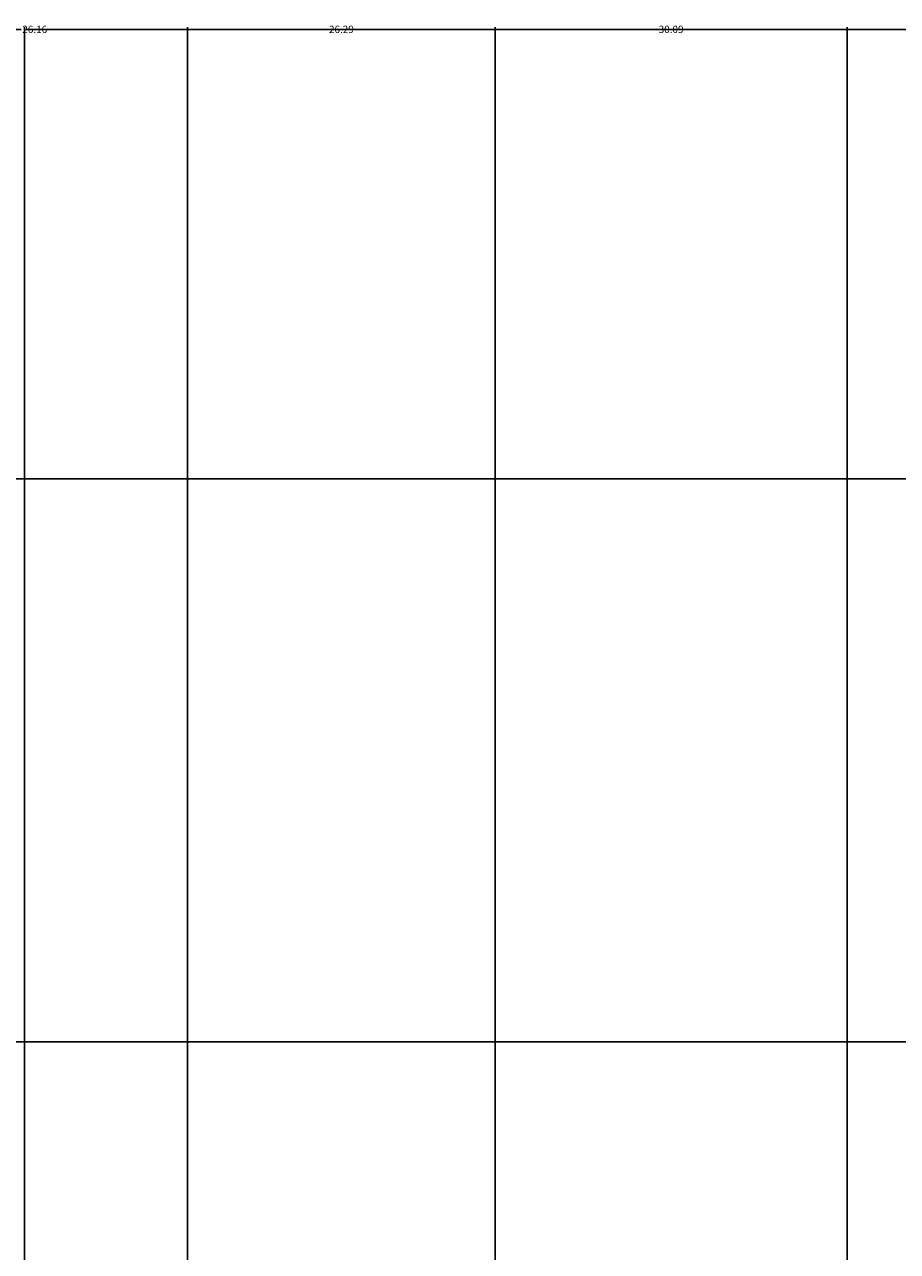
# Model space of a CAD drawing. Units: inches. Extents: x -13 to 809, y 112 to 656.
# Tile 31 of 55: x 107 to 182, y 551 to 656. Entities that reach past the tile are written whole.
import ezdxf

# ---------------------------------------------------------------- set-up
doc = ezdxf.new("R2010")
doc.units = ezdxf.units.IN
doc.header["$MEASUREMENT"] = 0
doc.layers.add('A-ANNO-DIMS', color=2, linetype='Continuous', lineweight=18)
doc.styles.get("Standard").update_dxf_attribs({"font": 'arial.ttf'})
doc.dimstyles.get("Standard").update_dxf_attribs({"dimtxt": 0.625, "dimasz": 0.18, "dimexe": 0.18, "dimexo": 0.0625, "dimgap": 0.09, "dimtad": 0, "dimtih": 1, "dimtoh": 1, "dimdec": 4, "dimzin": 0, "dimdsep": 46, "dimlunit": 4, "dimtxsty": 'Standard', "dimcen": 0.09, "dimadec": 0, "dimazin": 0, "dimtfac": 1, "dimtdec": 4, "dimtofl": 0, "dimtmove": 0, "dimatfit": 3, "dimfxl": 1, "dimtolj": 1, "dimtzin": 0, "dimarcsym": 0})

# ---------------------------------------------------------------- blocks, each defined once
blk = doc.blocks.new('*D23')
at = {"layer": 'A-ANNO-DIMS', "color": 0, "lineweight": -2, "transparency": 16777216}
for p, q in [((107.26, 510.58), (107.26, 655.96)), ((107.44, 655.78), (198.73, 655.78)), ((292.74, 655.78), (201.45, 655.78)), ((292.92, 569.3), (292.92, 655.96))]:
    blk.add_line(p, q, dxfattribs=at)
at = {"layer": 'A-ANNO-DIMS', "color": 0, "transparency": 16777216}
for points in [[(107.44, 655.81), (107.44, 655.75), (107.26, 655.78)], [(292.74, 655.81), (292.74, 655.75), (292.92, 655.78)]]:
    blk.add_solid(points, dxfattribs=at)
at = {"layer": 'Defpoints', "color": 0, "transparency": 16777216}
for p in [(292.92, 655.78), (292.92, 569.24), (107.26, 510.52)]:
    blk.add_point(p, dxfattribs=at)
at = {"layer": 'A-ANNO-DIMS', "color": 0, "transparency": 16777216, "insert": (200.09, 655.78), "char_height": 0.625, "attachment_point": 5}
blk.add_mtext('\\A1;185.66', dxfattribs=at)
blk = doc.blocks.new('*D36')
at = {"layer": 'A-ANNO-DIMS', "color": 0, "lineweight": -2, "transparency": 16777216}
for p, q in [((311.64, 569.24), (-12.1, 569.24)), ((-11.92, 569.06), (-11.92, 540.29)), ((-11.92, 510.7), (-11.92, 539.47)), ((107.2, 510.52), (-12.1, 510.52))]:
    blk.add_line(p, q, dxfattribs=at)
at = {"layer": 'A-ANNO-DIMS', "color": 0, "transparency": 16777216}
for points in [[(-11.95, 569.06), (-11.89, 569.06), (-11.92, 569.24)], [(-11.95, 510.7), (-11.89, 510.7), (-11.92, 510.52)]]:
    blk.add_solid(points, dxfattribs=at)
at = {"layer": 'Defpoints', "color": 0, "transparency": 16777216}
for p in [(-11.92, 569.24), (311.7, 569.24), (107.26, 510.52)]:
    blk.add_point(p, dxfattribs=at)
at = {"layer": 'A-ANNO-DIMS', "color": 0, "transparency": 16777216, "insert": (-11.92, 539.88), "char_height": 0.625, "attachment_point": 5}
blk.add_mtext('\\A1;58.72', dxfattribs=at)
blk = doc.blocks.new('*D37')
at = {"layer": 'A-ANNO-DIMS', "color": 0, "lineweight": -2, "transparency": 16777216}
for p, q in [((311.64, 617.37), (-12.1, 617.37)), ((-11.92, 617.19), (-11.92, 593.72)), ((-11.92, 569.42), (-11.92, 592.9)), ((311.64, 569.24), (-12.1, 569.24))]:
    blk.add_line(p, q, dxfattribs=at)
at = {"layer": 'A-ANNO-DIMS', "color": 0, "transparency": 16777216}
for points in [[(-11.95, 617.19), (-11.89, 617.19), (-11.92, 617.37)], [(-11.95, 569.42), (-11.89, 569.42), (-11.92, 569.24)]]:
    blk.add_solid(points, dxfattribs=at)
at = {"layer": 'Defpoints', "color": 0, "transparency": 16777216}
for p in [(-11.92, 617.37), (311.7, 617.37), (311.7, 569.24)]:
    blk.add_point(p, dxfattribs=at)
at = {"layer": 'A-ANNO-DIMS', "color": 0, "transparency": 16777216, "insert": (-11.92, 593.31), "char_height": 0.625, "attachment_point": 5}
blk.add_mtext('\\A1;48.13', dxfattribs=at)
blk = doc.blocks.new('*D95')
at = {"layer": 'A-ANNO-DIMS', "color": 0, "lineweight": -2, "transparency": 16777216}
for p, q in [((95.05, 462.58), (95.05, 655.96)), ((95.23, 655.78), (106.98, 655.78)), ((121.02, 655.78), (109.28, 655.78)), ((121.2, 452.63), (121.2, 655.96))]:
    blk.add_line(p, q, dxfattribs=at)
at = {"layer": 'A-ANNO-DIMS', "color": 0, "transparency": 16777216}
for points in [[(95.23, 655.81), (95.23, 655.75), (95.05, 655.78)], [(121.02, 655.81), (121.02, 655.75), (121.2, 655.78)]]:
    blk.add_solid(points, dxfattribs=at)
at = {"layer": 'Defpoints', "color": 0, "transparency": 16777216}
for p in [(121.2, 655.78), (95.05, 462.52), (121.2, 452.56)]:
    blk.add_point(p, dxfattribs=at)
at = {"layer": 'A-ANNO-DIMS', "color": 0, "transparency": 16777216, "insert": (108.13, 655.78), "char_height": 0.625, "attachment_point": 5}
blk.add_mtext('\\A1;26.16', dxfattribs=at)
blk = doc.blocks.new('*D96')
at = {"layer": 'A-ANNO-DIMS', "color": 0, "lineweight": -2, "transparency": 16777216}
for p, q in [((121.2, 452.63), (121.2, 655.96)), ((121.38, 655.78), (133.2, 655.78)), ((147.31, 655.78), (135.5, 655.78)), ((147.49, 452.63), (147.49, 655.96))]:
    blk.add_line(p, q, dxfattribs=at)
at = {"layer": 'A-ANNO-DIMS', "color": 0, "transparency": 16777216}
for points in [[(121.38, 655.81), (121.38, 655.75), (121.2, 655.78)], [(147.31, 655.81), (147.31, 655.75), (147.49, 655.78)]]:
    blk.add_solid(points, dxfattribs=at)
at = {"layer": 'Defpoints', "color": 0, "transparency": 16777216}
for p in [(147.49, 655.78), (121.2, 452.56), (147.49, 452.56)]:
    blk.add_point(p, dxfattribs=at)
at = {"layer": 'A-ANNO-DIMS', "color": 0, "transparency": 16777216, "insert": (134.35, 655.78), "char_height": 0.625, "attachment_point": 5}
blk.add_mtext('\\A1;26.29', dxfattribs=at)
blk = doc.blocks.new('*D97')
at = {"layer": 'A-ANNO-DIMS', "color": 0, "lineweight": -2, "transparency": 16777216}
for p, q in [((147.49, 452.63), (147.49, 655.96)), ((147.67, 655.78), (161.39, 655.78)), ((177.41, 655.78), (163.68, 655.78)), ((177.59, 452.63), (177.59, 655.96))]:
    blk.add_line(p, q, dxfattribs=at)
at = {"layer": 'A-ANNO-DIMS', "color": 0, "transparency": 16777216}
for points in [[(147.67, 655.81), (147.67, 655.75), (147.49, 655.78)], [(177.41, 655.81), (177.41, 655.75), (177.59, 655.78)]]:
    blk.add_solid(points, dxfattribs=at)
at = {"layer": 'Defpoints', "color": 0, "transparency": 16777216}
for p in [(177.59, 655.78), (147.49, 452.56), (177.59, 452.56)]:
    blk.add_point(p, dxfattribs=at)
at = {"layer": 'A-ANNO-DIMS', "color": 0, "transparency": 16777216, "insert": (162.54, 655.78), "char_height": 0.625, "attachment_point": 5}
blk.add_mtext('\\A1;30.09', dxfattribs=at)
blk = doc.blocks.new('*D98')
at = {"layer": 'A-ANNO-DIMS', "color": 0, "lineweight": -2, "transparency": 16777216}
for p, q in [((177.59, 452.63), (177.59, 655.96)), ((177.77, 655.78), (189.7, 655.78)), ((204.42, 655.78), (192.49, 655.78)), ((204.6, 452.63), (204.6, 655.96))]:
    blk.add_line(p, q, dxfattribs=at)
at = {"layer": 'A-ANNO-DIMS', "color": 0, "transparency": 16777216}
for points in [[(177.77, 655.81), (177.77, 655.75), (177.59, 655.78)], [(204.42, 655.81), (204.42, 655.75), (204.6, 655.78)]]:
    blk.add_solid(points, dxfattribs=at)
at = {"layer": 'Defpoints', "color": 0, "transparency": 16777216}
for p in [(204.6, 655.78), (177.59, 452.56), (204.6, 452.56)]:
    blk.add_point(p, dxfattribs=at)
at = {"layer": 'A-ANNO-DIMS', "color": 0, "transparency": 16777216, "insert": (191.09, 655.78), "char_height": 0.625, "attachment_point": 5}
blk.add_mtext('\\A1;27.017', dxfattribs=at)

msp = doc.modelspace()

# ---------------------------------------------------------------- dimensions: what is measured, and where the dimension line sits
at = {"layer": 'A-ANNO-DIMS'}
for base, p1, p2, override, picture, middle in [((121.2048, 655.7828), (95.0469, 462.5199), (121.2048, 452.5629), {"dimdec": 2, "dimlfac": 1, "dimrnd": 0, "dimzin": 0, "dimdsep": 46, "dimlunit": 2}, '*D95', (108.1258, 655.7828)), ((292.923, 655.7828), (107.2588, 510.5199), (292.923, 569.2414), {"dimdec": 2, "dimlfac": 1, "dimrnd": 0, "dimzin": 0, "dimdsep": 46, "dimlunit": 2}, '*D23', (200.0909, 655.7828)), ((147.4935, 655.7828), (121.2048, 452.5629), (147.4935, 452.5629), {"dimdec": 2, "dimlfac": 1, "dimrnd": 0, "dimzin": 0, "dimdsep": 46, "dimlunit": 2}, '*D96', (134.3491, 655.7828)), ((177.5857, 655.7828), (147.4935, 452.5629), (177.5857, 452.5629), {"dimdec": 2, "dimlfac": 1, "dimrnd": 0, "dimzin": 0, "dimdsep": 46, "dimlunit": 2}, '*D97', (162.5396, 655.7828)), ((204.6029, 655.7828), (177.5857, 452.5629), (204.6029, 452.5629), {"dimdec": 3, "dimlfac": 1, "dimrnd": 0, "dimzin": 0, "dimdsep": 46, "dimlunit": 2}, '*D98', (191.0943, 655.7828))]:
    dim = msp.add_linear_dim(base=base, p1=p1, p2=p2, dimstyle='Standard', override=override, dxfattribs=at)
    dim.commit()
    dim.dimension.update_dxf_attribs({"geometry": picture, "text_midpoint": middle})
for base, p1, p2, picture, middle in [((-11.9191, 617.3708), (311.6991, 569.2414), (311.6991, 617.3708), '*D37', (-11.9191, 593.3061)), ((-11.9191, 569.2414), (107.2588, 510.5199), (311.6991, 569.2414), '*D36', (-11.9191, 539.8806))]:
    dim = msp.add_linear_dim(base=base, p1=p1, p2=p2, angle=90, dimstyle='Standard', override={"dimdec": 2, "dimlfac": 1, "dimrnd": 0, "dimzin": 0, "dimdsep": 46, "dimlunit": 2}, dxfattribs=at)
    dim.commit()
    dim.dimension.update_dxf_attribs({"geometry": picture, "text_midpoint": middle})

doc.saveas('drawing.dxf')
